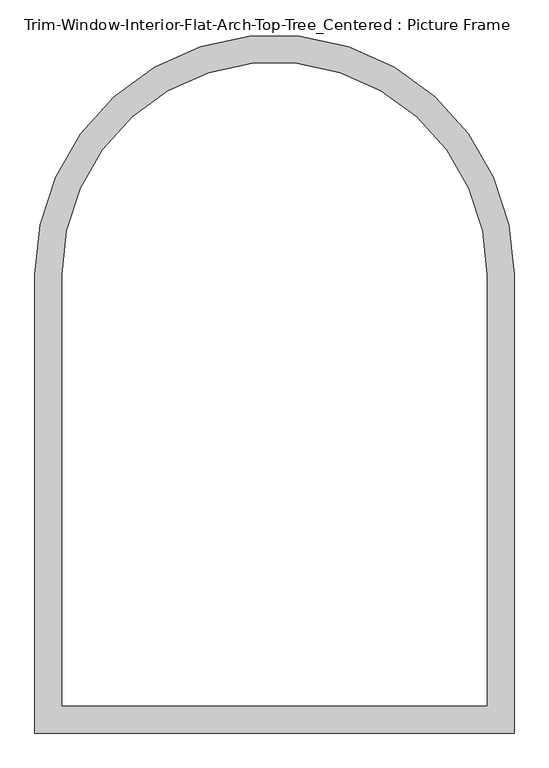
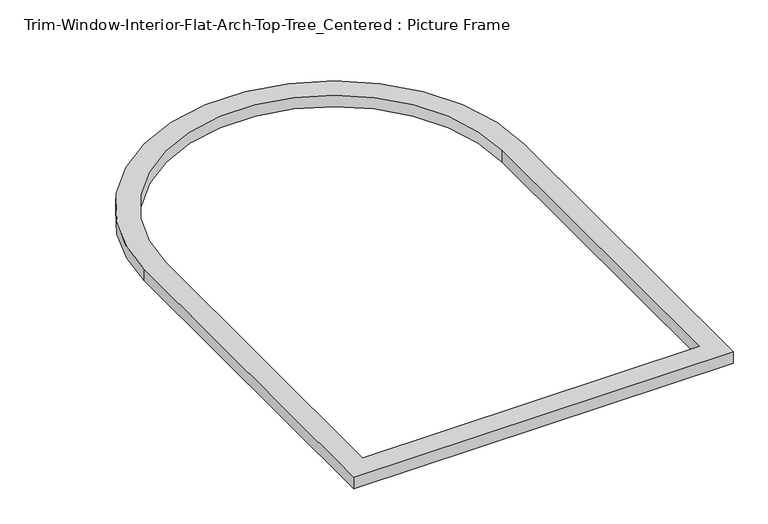
"""IFC4 building model written with IfcOpenShell, lengths in millimetres: proxy geometry, Trim-Window-Interior-Flat-Arch-Top-Tree_Centered : Picture Frame."""

from ifc_helpers import new_model, si_unit, point, frame_2d, origin, origin_with_axes, place, context, project, spatial, polyline, circle_curve, trimmed, segment, composite_curve, outline, extrude, source, transform, mapped, element, save


def trim_window_interior_flat_arch_top_tree_centered_picture_e2e46177(model_context):
    return source(origin(), model_context, "Body", "SweptSolid", [
        extrude(outline(composite_curve([segment(trimmed(circle_curve(frame_2d((0.0, -457.2)), 501.65), [point((-501.65, -457.2))], [point((501.65, -457.2))], False, "CARTESIAN"), True, "CONTINUOUS"), segment(polyline([(501.65, -457.2), (501.65, -1416.05), (-501.65, -1416.05), (-501.65, -457.2)]), True, "CONTINUOUS")], self_intersect=False), holes=[composite_curve([segment(polyline([(-444.5, -457.2), (-444.5, -1358.9), (444.5, -1358.9), (444.5, -457.2)]), True, "CONTINUOUS"), segment(trimmed(circle_curve(frame_2d((0.0, -457.2)), 444.5), [point((444.5, -457.2))], [point((-444.5, -457.2))], True, "CARTESIAN"), True, "CONTINUOUS")], self_intersect=False)]), origin_with_axes(), (0.0, 0.0, 1.0), 31.75),
    ])


if __name__ == "__main__":
    model = new_model("IFC4")
    model_context = context("Model", 3, world=origin())
    ifc_project = project(units=[si_unit("LENGTHUNIT", "METRE", prefix="MILLI")], contexts=[model_context])
    site = spatial("IfcSite", under=ifc_project)
    building = spatial("IfcBuilding", under=site)
    placement = place(None, origin())
    trim_window_interior_flat_arch_top_tree_centered_picture_shape = trim_window_interior_flat_arch_top_tree_centered_picture_e2e46177(model_context)
    element("IfcBuildingElementProxy", 1, Name="Trim-Window-Interior-Flat-Arch-Top-Tree_Centered : Picture Frame", ObjectType="Trim-Window-Interior-Flat-Arch-Top-Tree_Centered : Picture Frame", at=placement, inside=building, context=model_context, shape_type="MappedRepresentation", body=[
        mapped(trim_window_interior_flat_arch_top_tree_centered_picture_shape, transform((0.0, 0.0, 0.0), x_axis=(1.0, 0.0, 0.0), y_axis=(0.0, 1.0, 0.0), z_axis=(0.0, 0.0, 1.0))),
    ])
    save(model, "model.ifc")

# Revit data of these elements
# Type "Trim-Window-Interior-Flat-Arch-Top-Tree_Centered : Picture Frame"
#   Trim Thickness_Picture Frame = 0' - 1 1/4"
#   Trim Width = 0' - 2 1/4"
#   Trim Thickness_with Sill = 0' - 0 3/4"
#   Sill Thickness = 0' - 1 1/4"
#   Opening Width [instance default] = 2' - 0"
#   Opening Height [instance default] = 3' - 0"
#   Default Elevation = 4' - 0"
#   Sill = no
#   Picture Frame = yes
#   Trim Material [instance default] = none
# Element 1 (IfcBuildingElementProxy, "Trim-Window-Interior-Flat-Arch-Top-Tree_Centered : Picture Frame")
#   Opening Width = 3' - 0"
#   Opening Height = 4' - 6"
#   Trim Material = Wood - Stained
#   Materials on its faces: "Wood - Stained"
# Materials
#   "Wood - Stained": class "Wood", colour RGB 224 178 126, transparency 0, Cost = 0
